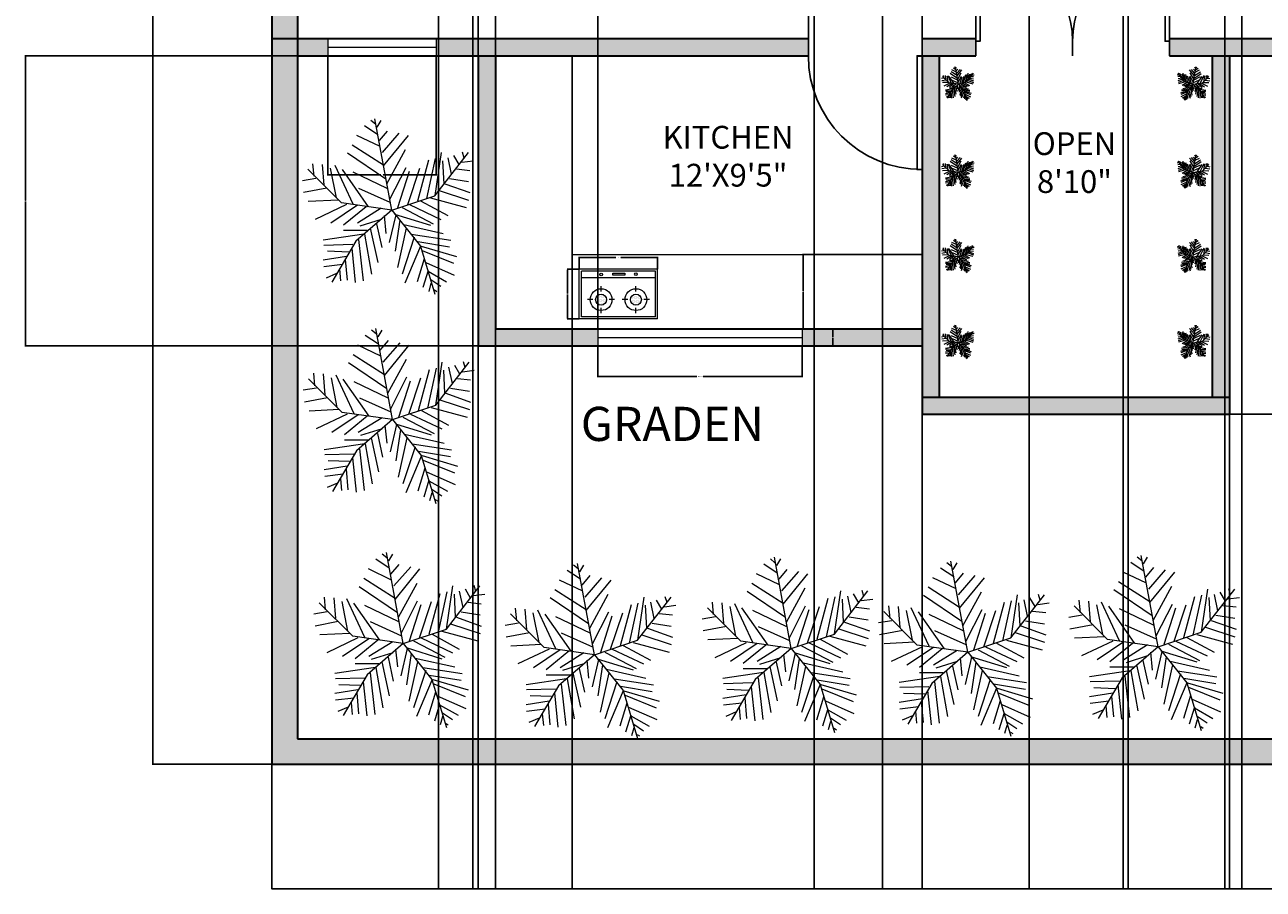
# Model space of a CAD drawing. Units: inches. Extents: x -89 to 661, y -827 to 77.
# Tile 1 of 5: x -89 to 347, y -827 to -523. Entities that reach past the tile are written whole.
import ezdxf

# ---------------------------------------------------------------- set-up
doc = ezdxf.new("R2010")
doc.units = ezdxf.units.IN
doc.header["$MEASUREMENT"] = 0
for name, color, linetype, lineweight in [('A-ANNO-DIMS', 2, 'Continuous', 18), ('A-ANNO-TEXT', 7, 'Continuous', 18), ('A-AREA-IDEN', 7, 'Continuous', 18), ('A-EQPM', 34, 'Continuous', 18), ('A-FLOR-CASE', 34, 'Continuous', 18), ('A-GLAZ', 5, 'Continuous', 18), ('A-WALL', 7, 'Continuous', 35), ('A-WALL-PATT', 30, 'Continuous', 13), ('DOOR', 5, 'Continuous', 25), ('TREE', 3, 'Continuous', 13)]:
    doc.layers.add(name, color=color, linetype=linetype, lineweight=lineweight)
doc.styles.get("Standard").update_dxf_attribs({"font": 'arial.ttf'})
doc.dimstyles.get("Standard").update_dxf_attribs({"dimtxt": 0.18, "dimasz": 0.18, "dimexe": 0.18, "dimexo": 0.0625, "dimgap": 0.09, "dimtad": 0, "dimtih": 1, "dimtoh": 1, "dimdec": 4, "dimzin": 0, "dimdsep": 46, "dimtxsty": 'Standard', "dimcen": 0.09, "dimadec": 0, "dimazin": 0, "dimtfac": 1, "dimtdec": 4, "dimtofl": 0, "dimtmove": 0, "dimatfit": 3, "dimfxl": 1, "dimtolj": 1, "dimtzin": 0, "dimarcsym": 0})

# ---------------------------------------------------------------- blocks, each defined once
blk = doc.blocks.new('*U5')
for p, q in [((-10.186, 53.64), (-13.084, 55.962)), ((0, 0), (-10.5, 57)), ((-9.099, 51.782), (-6.563, 55.962)), ((-7.288, 39.707), (-21.778, 46.673)), ((-8.737, 47.138), (-17.069, 52.711)), ((-7.65, 43.423), (-2.578, 49.46)), ((-5.839, 35.992), (4.667, 48.067)), ((-5.114, 27.632), (10.463, 46.673)), ((-5.114, 28.097), (-24.676, 40.636)), ((-3.665, 19.273), (-27.574, 35.527)), ((-2.941, 16.486), (8.652, 37.85)), ((16.259, 5.805), (23.142, 31.348)), ((22.055, 7.198), (27.489, 32.277)), ((27, 9), (48, 36)), ((27.127, 9.056), (31.112, 35.992)), ((35.096, 32.741), (37.27, 22.524)), ((38.719, 34.134), (41.979, 28.561)), ((44.153, 36.456), (45.239, 32.741)), ((-31.5, 4.5), (-52.5, 25.5)), ((-48.585, 21.131), (-49.309, 29.026)), ((-43.513, 28.561), (-42.427, 15.558)), ((-38.442, 26.239), (-34.819, 7.663)), ((-35.544, 28.097), (-24.314, 3.947)), ((-14.533, 2.09), (-30.834, 25.31)), ((-24.314, 23.917), (-2.941, 13.7)), ((-1.129, 6.734), (9.014, 26.704)), ((3.942, 1.625), (11.187, 24.381)), ((10.101, 3.483), (17.708, 26.239)), ((31.836, 30.883), (32.561, 16.486)), ((40.53, 25.775), (48.862, 24.846)), ((43.791, 29.954), (51.036, 30.883)), ((-47.498, 19.737), (-55.83, 18.344)), ((33.285, 16.486), (48.862, 10.913)), ((36.183, 19.737), (48.137, 17.88)), ((-40.615, 13.7), (-55.105, 10.913)), ((-20.691, 13.7), (-1.129, 4.876)), ((0, 0), (27, 9)), ((29.662, 12.307), (48.137, 6.269)), ((-33.37, 6.269), (-52.207, 5.34)), ((-28.299, 3.483), (-47.86, -5.805)), ((-21.416, 3.018), (-38.079, -8.128)), ((0, 0), (-31.5, 4.5)), ((-15.982, 2.09), (-30.11, -9.521)), ((0, 0), (-22.5, -19.5)), ((-6.563, 1.161), (-21.416, -8.128)), ((0, 0), (18, -22.5)), ((6.478, 1.625), (26.04, -8.592)), ((11.187, 3.483), (30.749, -5.805)), ((18.07, 5.805), (35.096, -3.483)), ((24.229, 7.663), (46.688, 1.625)), ((-6.563, -5.805), (-19.967, -9.985)), ((-4.752, -3.483), (-3.665, -14.629)), ((2.493, -3.019), (-1.491, -20.202)), ((1.769, -2.555), (24.229, -9.521)), ((5.029, -6.27), (2.131, -25.775)), ((-17.431, -15.094), (-42.789, -18.809)), ((-15.257, -12.772), (-30.11, -12.772)), ((-17.069, -15.094), (-12.721, -40.172)), ((-13.446, -11.378), (-8.737, -32.741)), ((-9.461, -8.592), (-6.201, -23.453)), ((9.014, -11.378), (3.58, -35.992)), ((7.565, -9.056), (32.198, -14.629)), ((12.274, -15.094), (36.907, -18.809)), ((-24.314, -21.596), (-42.427, -22.06)), ((-22.5, -19.5), (-37.5, -45)), ((-20.691, -18.345), (-17.793, -44.352)), ((14.085, -16.951), (6.478, -40.172)), ((18.07, -22.524), (8.289, -45.745)), ((16.259, -19.738), (36.183, -22.989)), ((18, -22.5), (27, -52.5)), ((18.433, -22.524), (40.53, -29.026)), ((-28.299, -29.026), (-42.789, -31.348)), ((-26.849, -26.24), (-40.253, -25.775)), ((-29.023, -30.884), (-27.936, -43.887)), ((-25.038, -23.918), (-22.865, -45.281)), ((20.244, -30.419), (15.897, -44.816)), ((19.157, -25.311), (38.719, -33.206)), ((-30.834, -34.135), (-42.427, -35.528)), ((-32.646, -36.921), (-31.921, -44.352)), ((22.78, -37.85), (19.519, -48.532)), ((21.331, -32.741), (39.081, -40.636)), ((22.78, -38.314), (34.372, -44.816)), ((-34.457, -39.708), (-40.978, -42.494)), ((24.591, -45.745), (23.142, -50.854)), ((24.591, -43.423), (30.749, -47.603)), ((26.764, -49.925), (28.213, -50.854))]:
    blk.add_line(p, q)
blk = doc.blocks.new('*U7')
for p, q in [((0, 0), (0, -6)), ((40, 0), (40, -6))]:
    blk.add_line(p, q)
blk.add_lwpolyline([(0, 0), (0, 40), (1.75, 40), (1.75, 0)], close=True)
blk.add_arc((0, 0), 40, 0, 90)
blk = doc.blocks.new('A$C475E21CF')
for p, q in [((0, 444), (0, 0)), ((0, 444), (700, 444)), ((700, 444), (700, 0)), ((19, 425), (19, 19)), ((19, 425), (680, 425)), ((194, 394), (194, 345)), ((505, 394), (505, 345)), ((680, 425), (680, 19)), ((73, 272), (122, 272)), ((149, 264), (149, 264)), ((155, 276), (155, 276)), ((155, 252), (155, 252)), ((161, 288), (161, 288)), ((161, 264), (161, 264)), ((161, 240), (161, 240)), ((167, 301), (167, 301)), ((167, 276), (167, 276)), ((167, 252), (167, 252)), ((173, 288), (173, 288)), ((173, 264), (173, 264)), ((173, 240), (173, 240)), ((179, 301), (179, 301)), ((179, 276), (179, 276)), ((179, 252), (179, 252)), ((179, 228), (179, 228)), ((185, 313), (185, 313)), ((185, 288), (185, 288)), ((185, 264), (185, 264)), ((185, 240), (185, 240)), ((191, 301), (191, 301)), ((191, 276), (191, 276)), ((191, 252), (191, 252)), ((191, 228), (191, 228)), ((197, 313), (197, 313)), ((197, 288), (197, 288)), ((197, 264), (197, 264)), ((197, 240), (197, 240)), ((203, 301), (203, 301)), ((203, 276), (203, 276)), ((203, 252), (203, 252)), ((203, 228), (203, 228)), ((209, 313), (209, 313)), ((209, 288), (209, 288)), ((209, 264), (209, 264)), ((209, 240), (209, 240)), ((216, 301), (216, 301)), ((216, 276), (216, 276)), ((216, 252), (216, 252)), ((216, 228), (216, 228)), ((222, 288), (222, 288)), ((222, 264), (222, 264)), ((222, 240), (222, 240)), ((228, 301), (228, 301)), ((228, 276), (228, 276)), ((228, 252), (228, 252)), ((234, 288), (234, 288)), ((234, 264), (234, 264)), ((234, 240), (234, 240)), ((240, 276), (240, 276)), ((240, 252), (240, 252)), ((267, 272), (316, 272)), ((384, 272), (433, 272)), ((462, 268), (462, 268)), ((468, 280), (468, 280)), ((468, 256), (468, 256)), ((474, 292), (474, 292)), ((474, 268), (474, 268)), ((474, 244), (474, 244)), ((480, 304), (480, 304)), ((480, 280), (480, 280)), ((480, 256), (480, 256)), ((486, 292), (486, 292)), ((486, 268), (486, 268)), ((486, 244), (486, 244)), ((492, 304), (492, 304)), ((492, 280), (492, 280)), ((492, 256), (492, 256)), ((492, 232), (492, 232)), ((498, 317), (498, 317)), ((498, 292), (498, 292)), ((498, 268), (498, 268)), ((498, 244), (498, 244)), ((505, 304), (505, 304)), ((505, 280), (505, 280)), ((505, 256), (505, 256)), ((505, 232), (505, 232)), ((511, 317), (511, 317)), ((511, 292), (511, 292)), ((511, 268), (511, 268)), ((511, 244), (511, 244)), ((517, 304), (517, 304)), ((517, 280), (517, 280)), ((517, 256), (517, 256)), ((517, 232), (517, 232)), ((523, 317), (523, 317)), ((523, 292), (523, 292)), ((523, 268), (523, 268)), ((523, 244), (523, 244)), ((529, 304), (529, 304)), ((529, 280), (529, 280)), ((529, 256), (529, 256)), ((529, 232), (529, 232)), ((535, 292), (535, 292)), ((535, 268), (535, 268)), ((535, 244), (535, 244)), ((541, 304), (541, 304)), ((541, 280), (541, 280)), ((541, 256), (541, 256)), ((547, 292), (547, 292)), ((547, 268), (547, 268)), ((547, 244), (547, 244)), ((553, 280), (553, 280)), ((553, 256), (553, 256)), ((578, 272), (627, 272)), ((194, 199), (194, 151)), ((505, 199), (505, 151)), ((0, 0), (700, 0)), ((19, 78), (680, 78)), ((19, 19), (680, 19)), ((293, 52), (401, 52)), ((293, 36), (293, 52)), ((401, 36), (293, 36)), ((401, 52), (401, 36))]:
    blk.add_line(p, q)
for centre, radius in [((194, 272), 97.2), ((505, 272), 97.2), ((194, 272), 48.6), ((505, 272), 48.6), ((194, 45), 11.7), ((505, 48), 11.7)]:
    blk.add_circle(centre, radius)
blk = doc.blocks.new('WIN-72-NOM')
for p, q in [((0, 6), (0, 0)), ((0, 6), (71.86, 6)), ((71.86, 6), (71.86, 0)), ((0, 3), (71.86, 3)), ((0, 0), (71.86, 0))]:
    blk.add_line(p, q)
blk = doc.blocks.new('*D19')
at = {"layer": 'A-ANNO-DIMS', "color": 0, "lineweight": -2, "transparency": 16777216}
for p, q in [((112.77, -636), (112.77, -646.9)), ((184.63, -636), (184.63, -646.9)), ((112.95, -646.72), (147.58, -646.72)), ((184.45, -646.72), (149.82, -646.72))]:
    blk.add_line(p, q, dxfattribs=at)
at = {"layer": 'A-ANNO-DIMS', "color": 0, "transparency": 16777216}
for points in [[(112.95, -646.69), (112.95, -646.75), (112.77, -646.72)], [(184.45, -646.69), (184.45, -646.75), (184.63, -646.72)]]:
    blk.add_solid(points, dxfattribs=at)
at = {"layer": 'Defpoints', "color": 0, "transparency": 16777216}
for p in [(112.77, -635.94), (184.63, -635.94), (184.63, -646.72)]:
    blk.add_point(p, dxfattribs=at)
at = {"layer": 'A-ANNO-DIMS', "color": 0, "transparency": 16777216, "insert": (148.7, -646.72), "char_height": 0.18, "attachment_point": 5}
blk.add_mtext('\\A1;WINDOW 72 TYP.', dxfattribs=at)
blk = doc.blocks.new('*D20')
at = {"layer": 'A-ANNO-DIMS', "color": 0, "lineweight": -2, "transparency": 16777216}
for p, q in [((184.7, -629.94), (195.59, -629.94)), ((195.41, -630.12), (195.41, -632.76)), ((195.41, -635.76), (195.41, -633.12)), ((184.7, -635.94), (195.59, -635.94))]:
    blk.add_line(p, q, dxfattribs=at)
at = {"layer": 'A-ANNO-DIMS', "color": 0, "transparency": 16777216}
for points in [[(195.38, -630.12), (195.44, -630.12), (195.41, -629.94)], [(195.38, -635.76), (195.44, -635.76), (195.41, -635.94)]]:
    blk.add_solid(points, dxfattribs=at)
at = {"layer": 'Defpoints', "color": 0, "transparency": 16777216}
for p in [(184.63, -629.94), (195.41, -629.94), (184.63, -635.94)]:
    blk.add_point(p, dxfattribs=at)
at = {"layer": 'A-ANNO-DIMS', "color": 0, "transparency": 16777216, "insert": (195.41, -632.94), "char_height": 0.18, "attachment_point": 5}
blk.add_mtext('\\A1;6 TYP.', dxfattribs=at)
blk = doc.blocks.new('*D29')
at = {"layer": 'A-ANNO-DIMS', "color": 0, "lineweight": -2, "transparency": 16777216}
for p, q in [((106.27, -608.89), (106.27, -604.64)), ((106.45, -604.82), (119.17, -604.82)), ((133.64, -604.82), (120.93, -604.82)), ((133.82, -608.89), (133.82, -604.64))]:
    blk.add_line(p, q, dxfattribs=at)
at = {"layer": 'A-ANNO-DIMS', "color": 0, "transparency": 16777216}
for points in [[(106.45, -604.79), (106.45, -604.85), (106.27, -604.82)], [(133.64, -604.79), (133.64, -604.85), (133.82, -604.82)]]:
    blk.add_solid(points, dxfattribs=at)
at = {"layer": 'Defpoints', "color": 0, "transparency": 16777216}
for p in [(106.27, -604.82), (106.27, -608.95), (133.82, -608.95)]:
    blk.add_point(p, dxfattribs=at)
at = {"layer": 'A-ANNO-DIMS', "color": 0, "transparency": 16777216, "insert": (120.05, -604.82), "char_height": 0.18, "attachment_point": 5}
blk.add_mtext('\\A1;COOKTOP 28', dxfattribs=at)
blk = doc.blocks.new('*D30')
at = {"layer": 'A-ANNO-DIMS', "color": 0, "lineweight": -2, "transparency": 16777216}
for p, q in [((106.21, -608.95), (101.96, -608.95)), ((102.14, -609.13), (102.14, -617.52)), ((102.14, -626.27), (102.14, -617.88)), ((106.21, -626.45), (101.96, -626.45))]:
    blk.add_line(p, q, dxfattribs=at)
at = {"layer": 'A-ANNO-DIMS', "color": 0, "transparency": 16777216}
for points in [[(102.11, -609.13), (102.17, -609.13), (102.14, -608.95)], [(102.11, -626.27), (102.17, -626.27), (102.14, -626.45)]]:
    blk.add_solid(points, dxfattribs=at)
at = {"layer": 'Defpoints', "color": 0, "transparency": 16777216}
for p in [(106.27, -608.95), (102.14, -626.45), (106.27, -626.45)]:
    blk.add_point(p, dxfattribs=at)
at = {"layer": 'A-ANNO-DIMS', "color": 0, "transparency": 16777216, "insert": (102.14, -617.7), "char_height": 0.18, "attachment_point": 5}
blk.add_mtext('\\A1;17', dxfattribs=at)
blk = doc.blocks.new('*D31')
at = {"layer": 'A-ANNO-DIMS', "color": 0, "lineweight": -2, "transparency": 16777216}
for p, q in [((-1.81, -783), (-1.81, -826.85)), ((619.19, -783), (619.19, -826.85)), ((-1.63, -826.67), (308.41, -826.67)), ((619.01, -826.67), (308.96, -826.67))]:
    blk.add_line(p, q, dxfattribs=at)
at = {"layer": 'A-ANNO-DIMS', "color": 0, "transparency": 16777216}
for points in [[(-1.63, -826.64), (-1.63, -826.7), (-1.81, -826.67)], [(619.01, -826.64), (619.01, -826.7), (619.19, -826.67)]]:
    blk.add_solid(points, dxfattribs=at)
at = {"layer": 'Defpoints', "color": 0, "transparency": 16777216}
for p in [(-1.81, -782.94), (619.19, -782.94), (619.19, -826.67)]:
    blk.add_point(p, dxfattribs=at)
at = {"layer": 'A-ANNO-DIMS', "color": 0, "transparency": 16777216, "insert": (308.69, -826.67), "char_height": 0.18, "attachment_point": 5}
blk.add_mtext('\\A1;621', dxfattribs=at)
blk = doc.blocks.new('*D32')
at = {"layer": 'A-ANNO-DIMS', "color": 0, "lineweight": -2, "transparency": 16777216}
for p, q in [((-1.88, 29.06), (-43.85, 29.06)), ((-43.67, 28.88), (-43.67, -376.76)), ((-43.67, -782.76), (-43.67, -377.12)), ((-1.88, -782.94), (-43.85, -782.94))]:
    blk.add_line(p, q, dxfattribs=at)
at = {"layer": 'A-ANNO-DIMS', "color": 0, "transparency": 16777216}
for points in [[(-43.7, 28.88), (-43.64, 28.88), (-43.67, 29.06)], [(-43.7, -782.76), (-43.64, -782.76), (-43.67, -782.94)]]:
    blk.add_solid(points, dxfattribs=at)
at = {"layer": 'Defpoints', "color": 0, "transparency": 16777216}
for p in [(-43.67, 29.06), (-1.81, 29.06), (-1.81, -782.94)]:
    blk.add_point(p, dxfattribs=at)
at = {"layer": 'A-ANNO-DIMS', "color": 0, "transparency": 16777216, "insert": (-43.67, -376.94), "char_height": 0.18, "attachment_point": 5}
blk.add_mtext('\\A1;812', dxfattribs=at)
blk = doc.blocks.new('*D44')
at = {"layer": 'A-ANNO-DIMS', "color": 0, "lineweight": -2, "transparency": 16777216}
for p, q in [((299.19, -34), (299.19, -826.85)), ((333.19, -34), (333.19, -826.85)), ((299.37, -826.67), (315.97, -826.67)), ((333.01, -826.67), (316.4, -826.67))]:
    blk.add_line(p, q, dxfattribs=at)
at = {"layer": 'A-ANNO-DIMS', "color": 0, "transparency": 16777216}
for points in [[(299.37, -826.64), (299.37, -826.7), (299.19, -826.67)], [(333.01, -826.64), (333.01, -826.7), (333.19, -826.67)]]:
    blk.add_solid(points, dxfattribs=at)
at = {"layer": 'Defpoints', "color": 0, "transparency": 16777216}
for p in [(299.19, -33.94), (333.19, -33.94), (333.19, -826.67)]:
    blk.add_point(p, dxfattribs=at)
at = {"layer": 'A-ANNO-DIMS', "color": 0, "transparency": 16777216, "insert": (316.19, -826.67), "char_height": 0.18, "attachment_point": 5}
blk.add_mtext('\\A1;34', dxfattribs=at)
blk = doc.blocks.new('*D46')
at = {"layer": 'A-ANNO-DIMS', "color": 0, "lineweight": -2, "transparency": 16777216}
for p, q in [((333.19, -34), (333.19, -826.85)), ((339.19, -34), (339.19, -826.85)), ((333.37, -826.67), (336.04, -826.67)), ((339.01, -826.67), (336.34, -826.67))]:
    blk.add_line(p, q, dxfattribs=at)
at = {"layer": 'A-ANNO-DIMS', "color": 0, "transparency": 16777216}
for points in [[(333.37, -826.64), (333.37, -826.7), (333.19, -826.67)], [(339.01, -826.64), (339.01, -826.7), (339.19, -826.67)]]:
    blk.add_solid(points, dxfattribs=at)
at = {"layer": 'Defpoints', "color": 0, "transparency": 16777216}
for p in [(333.19, -33.94), (339.19, -33.94), (339.19, -826.67)]:
    blk.add_point(p, dxfattribs=at)
at = {"layer": 'A-ANNO-DIMS', "color": 0, "transparency": 16777216, "insert": (336.19, -826.67), "char_height": 0.18, "attachment_point": 5}
blk.add_mtext('\\A1;6', dxfattribs=at)
blk = doc.blocks.new('*D48')
at = {"layer": 'A-ANNO-DIMS', "color": 0, "lineweight": -2, "transparency": 16777216}
for p, q in [((297.44, 2.03), (297.44, -826.85)), ((264.44, -8.47), (264.44, -826.85)), ((264.62, -826.67), (280.72, -826.67)), ((297.26, -826.67), (281.15, -826.67))]:
    blk.add_line(p, q, dxfattribs=at)
at = {"layer": 'A-ANNO-DIMS', "color": 0, "transparency": 16777216}
for points in [[(264.62, -826.64), (264.62, -826.7), (264.44, -826.67)], [(297.26, -826.64), (297.26, -826.7), (297.44, -826.67)]]:
    blk.add_solid(points, dxfattribs=at)
at = {"layer": 'Defpoints', "color": 0, "transparency": 16777216}
for p in [(297.44, 2.09), (264.44, -8.41), (297.44, -826.67)]:
    blk.add_point(p, dxfattribs=at)
at = {"layer": 'A-ANNO-DIMS', "color": 0, "transparency": 16777216, "insert": (280.94, -826.67), "char_height": 0.18, "attachment_point": 5}
blk.add_mtext('\\A1;33', dxfattribs=at)
blk = doc.blocks.new('*D55')
at = {"layer": 'A-ANNO-DIMS', "color": 0, "lineweight": -2, "transparency": 16777216}
for p, q in [((56.84, -267), (56.84, -826.85)), ((68.84, -267), (68.84, -826.85)), ((57.02, -826.67), (62.63, -826.67)), ((68.66, -826.67), (63.05, -826.67))]:
    blk.add_line(p, q, dxfattribs=at)
at = {"layer": 'A-ANNO-DIMS', "color": 0, "transparency": 16777216}
for points in [[(57.02, -826.64), (57.02, -826.7), (56.84, -826.67)], [(68.66, -826.64), (68.66, -826.7), (68.84, -826.67)]]:
    blk.add_solid(points, dxfattribs=at)
at = {"layer": 'Defpoints', "color": 0, "transparency": 16777216}
for p in [(56.84, -266.94), (68.84, -266.94), (68.84, -826.67)]:
    blk.add_point(p, dxfattribs=at)
at = {"layer": 'A-ANNO-DIMS', "color": 0, "transparency": 16777216, "insert": (62.84, -826.67), "char_height": 0.18, "attachment_point": 5}
blk.add_mtext('\\A1;12', dxfattribs=at)
blk = doc.blocks.new('*D56')
at = {"layer": 'A-ANNO-DIMS', "color": 0, "lineweight": -2, "transparency": 16777216}
for p, q in [((188.84, -312), (188.84, -826.85)), ((212.84, -318), (212.84, -826.85)), ((189.02, -826.67), (200.62, -826.67)), ((212.66, -826.67), (201.06, -826.67))]:
    blk.add_line(p, q, dxfattribs=at)
at = {"layer": 'A-ANNO-DIMS', "color": 0, "transparency": 16777216}
for points in [[(189.02, -826.64), (189.02, -826.7), (188.84, -826.67)], [(212.66, -826.64), (212.66, -826.7), (212.84, -826.67)]]:
    blk.add_solid(points, dxfattribs=at)
at = {"layer": 'Defpoints', "color": 0, "transparency": 16777216}
for p in [(188.84, -311.94), (212.84, -317.94), (212.84, -826.67)]:
    blk.add_point(p, dxfattribs=at)
at = {"layer": 'A-ANNO-DIMS', "color": 0, "transparency": 16777216, "insert": (200.84, -826.67), "char_height": 0.18, "attachment_point": 5}
blk.add_mtext('\\A1;24', dxfattribs=at)
blk = doc.blocks.new('*D57')
at = {"layer": 'A-ANNO-DIMS', "color": 0, "lineweight": -2, "transparency": 16777216}
for p, q in [((70.79, -636), (70.79, -826.85)), ((226.79, -636), (226.79, -826.85)), ((70.97, -826.67), (148.51, -826.67)), ((226.61, -826.67), (149.07, -826.67))]:
    blk.add_line(p, q, dxfattribs=at)
at = {"layer": 'A-ANNO-DIMS', "color": 0, "transparency": 16777216}
for points in [[(70.97, -826.64), (70.97, -826.7), (70.79, -826.67)], [(226.61, -826.64), (226.61, -826.7), (226.79, -826.67)]]:
    blk.add_solid(points, dxfattribs=at)
at = {"layer": 'Defpoints', "color": 0, "transparency": 16777216}
for p in [(70.79, -635.94), (226.79, -635.94), (226.79, -826.67)]:
    blk.add_point(p, dxfattribs=at)
at = {"layer": 'A-ANNO-DIMS', "color": 0, "transparency": 16777216, "insert": (148.79, -826.67), "char_height": 0.18, "attachment_point": 5}
blk.add_mtext('\\A1;156', dxfattribs=at)
blk = doc.blocks.new('*D58')
at = {"layer": 'A-ANNO-DIMS', "color": 0, "lineweight": -2, "transparency": 16777216}
for p, q in [((226.79, -660), (226.79, -826.85)), ((334.79, -660), (334.79, -826.85)), ((226.97, -826.67), (280.51, -826.67)), ((334.61, -826.67), (281.07, -826.67))]:
    blk.add_line(p, q, dxfattribs=at)
at = {"layer": 'A-ANNO-DIMS', "color": 0, "transparency": 16777216}
for points in [[(226.97, -826.64), (226.97, -826.7), (226.79, -826.67)], [(334.61, -826.64), (334.61, -826.7), (334.79, -826.67)]]:
    blk.add_solid(points, dxfattribs=at)
at = {"layer": 'Defpoints', "color": 0, "transparency": 16777216}
for p in [(226.79, -659.94), (334.79, -659.94), (334.79, -826.67)]:
    blk.add_point(p, dxfattribs=at)
at = {"layer": 'A-ANNO-DIMS', "color": 0, "transparency": 16777216, "insert": (280.79, -826.67), "char_height": 0.18, "attachment_point": 5}
blk.add_mtext('\\A1;108', dxfattribs=at)
blk = doc.blocks.new('*D59')
at = {"layer": 'A-ANNO-DIMS', "color": 0, "lineweight": -2, "transparency": 16777216}
for p, q in [((70.73, -533.94), (-88.61, -533.94)), ((-88.43, -534.12), (-88.43, -584.76)), ((-88.43, -635.76), (-88.43, -585.12)), ((70.73, -635.94), (-88.61, -635.94))]:
    blk.add_line(p, q, dxfattribs=at)
at = {"layer": 'A-ANNO-DIMS', "color": 0, "transparency": 16777216}
for points in [[(-88.46, -534.12), (-88.4, -534.12), (-88.43, -533.94)], [(-88.46, -635.76), (-88.4, -635.76), (-88.43, -635.94)]]:
    blk.add_solid(points, dxfattribs=at)
at = {"layer": 'Defpoints', "color": 0, "transparency": 16777216}
for p in [(-88.43, -533.94), (70.79, -533.94), (70.79, -635.94)]:
    blk.add_point(p, dxfattribs=at)
at = {"layer": 'A-ANNO-DIMS', "color": 0, "transparency": 16777216, "insert": (-88.43, -584.94), "char_height": 0.18, "attachment_point": 5}
blk.add_mtext('\\A1;102', dxfattribs=at)
blk = doc.blocks.new('*D60')
at = {"layer": 'A-ANNO-DIMS', "color": 0, "lineweight": -2, "transparency": 16777216}
for p, q in [((334.85, -533.94), (661.23, -533.94)), ((661.05, -534.12), (661.05, -596.76)), ((661.05, -659.76), (661.05, -597.12)), ((334.85, -659.94), (661.23, -659.94))]:
    blk.add_line(p, q, dxfattribs=at)
at = {"layer": 'A-ANNO-DIMS', "color": 0, "transparency": 16777216}
for points in [[(661.02, -534.12), (661.08, -534.12), (661.05, -533.94)], [(661.02, -659.76), (661.08, -659.76), (661.05, -659.94)]]:
    blk.add_solid(points, dxfattribs=at)
at = {"layer": 'Defpoints', "color": 0, "transparency": 16777216}
for p in [(334.79, -533.94), (661.05, -533.94), (334.79, -659.94)]:
    blk.add_point(p, dxfattribs=at)
at = {"layer": 'A-ANNO-DIMS', "color": 0, "transparency": 16777216, "insert": (661.05, -596.94), "char_height": 0.18, "attachment_point": 5}
blk.add_mtext('\\A1;126', dxfattribs=at)
blk = doc.blocks.new('*D62')
at = {"layer": 'A-ANNO-DIMS', "color": 0, "lineweight": -2, "transparency": 16777216}
for p, q in [((186.79, -527.88), (186.79, 77.13)), ((186.97, 76.95), (206.57, 76.95)), ((226.61, 76.95), (207.01, 76.95)), ((226.79, -527.88), (226.79, 77.13))]:
    blk.add_line(p, q, dxfattribs=at)
at = {"layer": 'A-ANNO-DIMS', "color": 0, "transparency": 16777216}
for points in [[(186.97, 76.98), (186.97, 76.92), (186.79, 76.95)], [(226.61, 76.98), (226.61, 76.92), (226.79, 76.95)]]:
    blk.add_solid(points, dxfattribs=at)
at = {"layer": 'Defpoints', "color": 0, "transparency": 16777216}
for p in [(226.79, 76.95), (186.79, -527.94), (226.79, -527.94)]:
    blk.add_point(p, dxfattribs=at)
at = {"layer": 'A-ANNO-DIMS', "color": 0, "transparency": 16777216, "insert": (206.79, 76.95), "char_height": 0.18, "attachment_point": 5}
blk.add_mtext('\\A1;40', dxfattribs=at)
blk = doc.blocks.new('*D63')
at = {"layer": 'A-ANNO-DIMS', "color": 0, "lineweight": -2, "transparency": 16777216}
for p, q in [((7.19, -533.88), (7.19, -491.9)), ((70.79, -533.88), (70.79, -491.9)), ((7.37, -492.08), (38.66, -492.08)), ((70.61, -492.08), (39.31, -492.08))]:
    blk.add_line(p, q, dxfattribs=at)
at = {"layer": 'A-ANNO-DIMS', "color": 0, "transparency": 16777216}
for points in [[(7.37, -492.05), (7.37, -492.11), (7.19, -492.08)], [(70.61, -492.05), (70.61, -492.11), (70.79, -492.08)]]:
    blk.add_solid(points, dxfattribs=at)
at = {"layer": 'Defpoints', "color": 0, "transparency": 16777216}
for p in [(70.79, -492.08), (7.19, -533.94), (70.79, -533.94)]:
    blk.add_point(p, dxfattribs=at)
at = {"layer": 'A-ANNO-DIMS', "color": 0, "transparency": 16777216, "insert": (38.99, -492.08), "char_height": 0.18, "attachment_point": 5}
blk.add_mtext('\\A1;63.6', dxfattribs=at)
blk = doc.blocks.new('*D66')
at = {"layer": 'A-ANNO-DIMS', "color": 0, "lineweight": -2, "transparency": 16777216}
for p, q in [((17.9, -534), (17.9, -575.98)), ((55.96, -534), (55.96, -575.98)), ((18.08, -575.8), (36.54, -575.8)), ((55.78, -575.8), (37.33, -575.8))]:
    blk.add_line(p, q, dxfattribs=at)
at = {"layer": 'A-ANNO-DIMS', "color": 0, "transparency": 16777216}
for points in [[(18.08, -575.77), (18.08, -575.83), (17.9, -575.8)], [(55.78, -575.77), (55.78, -575.83), (55.96, -575.8)]]:
    blk.add_solid(points, dxfattribs=at)
at = {"layer": 'Defpoints', "color": 0, "transparency": 16777216}
for p in [(17.9, -533.94), (55.96, -533.94), (17.9, -575.8)]:
    blk.add_point(p, dxfattribs=at)
at = {"layer": 'A-ANNO-DIMS', "color": 0, "transparency": 16777216, "insert": (36.93, -575.8), "char_height": 0.18, "attachment_point": 5}
blk.add_mtext('\\A1;38.06', dxfattribs=at)
blk = doc.blocks.new('*D67')
at = {"layer": 'A-ANNO-DIMS', "color": 0, "lineweight": -2, "transparency": 16777216}
for p, q in [((226.73, -603.76), (184.75, -603.76)), ((184.93, -603.94), (184.93, -616.67)), ((184.93, -629.76), (184.93, -617.03)), ((226.73, -629.94), (184.75, -629.94))]:
    blk.add_line(p, q, dxfattribs=at)
at = {"layer": 'A-ANNO-DIMS', "color": 0, "transparency": 16777216}
for points in [[(184.9, -603.94), (184.96, -603.94), (184.93, -603.76)], [(184.9, -629.76), (184.96, -629.76), (184.93, -629.94)]]:
    blk.add_solid(points, dxfattribs=at)
at = {"layer": 'Defpoints', "color": 0, "transparency": 16777216}
for p in [(184.93, -603.76), (226.79, -603.76), (226.79, -629.94)]:
    blk.add_point(p, dxfattribs=at)
at = {"layer": 'A-ANNO-DIMS', "color": 0, "transparency": 16777216, "insert": (184.93, -616.85), "char_height": 0.18, "attachment_point": 5}
blk.add_mtext('\\A1;26.18', dxfattribs=at)
blk = doc.blocks.new('*D68')
at = {"layer": 'A-ANNO-DIMS', "color": 0, "lineweight": -2, "transparency": 16777216}
for p, q in [((76.79, -534), (76.79, -826.85)), ((103.81, -534), (103.81, -826.85)), ((76.97, -826.67), (89.9, -826.67)), ((103.63, -826.67), (90.69, -826.67))]:
    blk.add_line(p, q, dxfattribs=at)
at = {"layer": 'A-ANNO-DIMS', "color": 0, "transparency": 16777216}
for points in [[(76.97, -826.64), (76.97, -826.7), (76.79, -826.67)], [(103.63, -826.64), (103.63, -826.7), (103.81, -826.67)]]:
    blk.add_solid(points, dxfattribs=at)
at = {"layer": 'Defpoints', "color": 0, "transparency": 16777216}
for p in [(76.79, -533.94), (103.81, -533.94), (103.81, -826.67)]:
    blk.add_point(p, dxfattribs=at)
at = {"layer": 'A-ANNO-DIMS', "color": 0, "transparency": 16777216, "insert": (90.3, -826.67), "char_height": 0.18, "attachment_point": 5}
blk.add_mtext('\\A1;27.02', dxfattribs=at)
blk = doc.blocks.new('*D69')
at = {"layer": 'A-ANNO-DIMS', "color": 0, "lineweight": -2, "transparency": 16777216}
for p, q in [((76.79, -629.88), (76.79, 77.13)), ((76.97, 76.95), (94.39, 76.95)), ((112.59, 76.95), (95.17, 76.95)), ((112.77, -629.88), (112.77, 77.13))]:
    blk.add_line(p, q, dxfattribs=at)
at = {"layer": 'A-ANNO-DIMS', "color": 0, "transparency": 16777216}
for points in [[(76.97, 76.98), (76.97, 76.92), (76.79, 76.95)], [(112.59, 76.98), (112.59, 76.92), (112.77, 76.95)]]:
    blk.add_solid(points, dxfattribs=at)
at = {"layer": 'Defpoints', "color": 0, "transparency": 16777216}
for p in [(112.77, 76.95), (76.79, -629.94), (112.77, -629.94)]:
    blk.add_point(p, dxfattribs=at)
at = {"layer": 'A-ANNO-DIMS', "color": 0, "transparency": 16777216, "insert": (94.78, 76.95), "char_height": 0.18, "attachment_point": 5}
blk.add_mtext('\\A1;35.98', dxfattribs=at)
blk = doc.blocks.new('*D74')
at = {"layer": 'A-ANNO-DIMS', "color": 0, "lineweight": -2, "transparency": 16777216}
for p, q in [((313.68, -527.88), (313.68, -485.9)), ((313.86, -486.08), (351.48, -486.08)), ((389.89, -486.08), (352.27, -486.08)), ((390.07, -527.88), (390.07, -485.9))]:
    blk.add_line(p, q, dxfattribs=at)
at = {"layer": 'A-ANNO-DIMS', "color": 0, "transparency": 16777216}
for points in [[(313.86, -486.05), (313.86, -486.11), (313.68, -486.08)], [(389.89, -486.05), (389.89, -486.11), (390.07, -486.08)]]:
    blk.add_solid(points, dxfattribs=at)
at = {"layer": 'Defpoints', "color": 0, "transparency": 16777216}
for p in [(390.07, -486.08), (313.68, -527.94), (390.07, -527.94)]:
    blk.add_point(p, dxfattribs=at)
at = {"layer": 'A-ANNO-DIMS', "color": 0, "transparency": 16777216, "insert": (351.88, -486.08), "char_height": 0.18, "attachment_point": 5}
blk.add_mtext('\\A1;76.39', dxfattribs=at)

msp = doc.modelspace()

# ---------------------------------------------------------------- hatches: boundary and pattern name
at = {"layer": 'A-WALL-PATT'}
h = msp.add_hatch(color=256, dxfattribs=at)
h.dxf.hatch_style = 1
h.paths.add_polyline_path([(255.186, 29.06), (-1.814, 29.06), (-1.814, -33.94), (7.186, -33.94), (7.186, -27.94), (7.186, 20.06), (255.186, 20.06)])
h.paths.add_polyline_path([(174.616, -27.94), (7.186, -27.94), (7.186, -33.94), (174.616, -33.94)], flags=17)
h.paths.add_polyline_path([(7.186, -33.94), (-1.814, -33.94), (-1.814, -527.94), (7.186, -527.94), (7.186, -425.94), (7.186, -311.94), (7.186, -207.94)])
h.paths.add_polyline_path([(7.186, -527.94), (-1.814, -527.94), (-1.814, -782.94), (430.186, -782.94), (430.186, -773.94), (7.186, -773.94)])
h = msp.add_hatch(color=256, dxfattribs=at)
h.dxf.hatch_style = 1
h.paths.add_polyline_path([(619.186, -533.94), (610.186, -533.94), (610.186, -773.94), (610.186, -782.94), (619.186, -782.94)])
h.paths.add_polyline_path([(610.186, -527.94), (461.934, -527.94), (461.934, -533.94), (610.186, -533.94)])
h.paths.add_polyline_path([(390.071, -527.94), (313.682, -527.94), (313.682, -528.84), (313.682, -533.94), (390.071, -533.94)])
h.paths.add_polyline_path([(334.788, -533.94), (328.788, -533.94), (328.788, -653.94), (334.788, -653.94)])
h.paths.add_polyline_path([(334.788, -653.94), (226.788, -653.94), (226.788, -659.94), (334.788, -659.94)])
h.paths.add_polyline_path([(232.788, -533.94), (226.788, -533.94), (226.788, -573.94), (226.788, -653.94), (232.788, -653.94)])
h.paths.add_polyline_path([(245.682, -528.84), (245.682, -527.94), (226.788, -527.94), (226.788, -533.94), (232.788, -533.94), (245.682, -533.94)])
h.paths.add_polyline_path([(226.788, -629.94), (184.634, -629.94), (184.634, -635.94), (226.788, -635.94)])
h.paths.add_polyline_path([(76.788, -533.94), (70.788, -533.94), (70.788, -635.94), (112.77, -635.94), (112.77, -629.94), (76.788, -629.94)])
h.paths.add_polyline_path([(186.788, -527.94), (55.963, -527.94), (55.963, -533.94), (186.788, -533.94)])
h.paths.add_polyline_path([(17.901, -527.94), (7.186, -527.94), (7.186, -533.94), (17.901, -533.94)])

# ---------------------------------------------------------------- linework, layer by layer
at = {"layer": 'A-FLOR-CASE'}
for p, q in [((103.806, -533.94), (103.806, -603.761)), ((103.806, -603.761), (226.788, -603.761))]:
    msp.add_line(p, q, dxfattribs=at)
at = {"layer": 'A-GLAZ'}
for p, q in [((17.901, -527.94), (17.901, -533.94)), ((17.901, -527.94), (55.963, -527.94)), ((17.901, -530.94), (55.963, -530.94)), ((55.963, -527.94), (55.963, -533.94)), ((17.901, -533.94), (55.963, -533.94))]:
    msp.add_line(p, q, dxfattribs=at)
at = {"layer": 'A-WALL'}
for p, q in [((-1.814, 29.06), (-1.814, -782.94)), ((7.186, -425.94), (7.186, -527.94)), ((-1.814, -527.94), (186.788, -527.94)), ((7.186, -527.94), (7.186, -773.94)), ((226.788, -527.94), (245.682, -527.94)), ((279.677, -527.94), (279.694, -527.94)), ((313.682, -527.94), (610.186, -527.94)), ((7.186, -533.94), (186.788, -533.94)), ((70.788, -533.94), (70.788, -635.94)), ((76.788, -533.94), (76.788, -629.94)), ((225.038, -533.94), (245.682, -533.94)), ((226.788, -533.94), (226.788, -659.94)), ((232.788, -533.94), (232.788, -653.94)), ((313.682, -533.94), (619.186, -533.94)), ((328.788, -533.94), (328.788, -653.94)), ((334.788, -533.94), (334.788, -659.94)), ((76.788, -629.94), (226.788, -629.94)), ((70.788, -635.94), (226.788, -635.94)), ((226.788, -653.94), (334.788, -653.94)), ((226.788, -659.94), (334.788, -659.94)), ((7.186, -773.94), (430.186, -773.94)), ((-1.814, -782.94), (430.186, -782.94))]:
    msp.add_line(p, q, dxfattribs=at)

# ---------------------------------------------------------------- block references
at = {"layer": 'A-EQPM', "xscale": 0.0393700787401575, "yscale": 0.0393700787401575, "zscale": 0.0393700787401575, "rotation": 180}
msp.add_blockref('A$C475E21CF', (133.825, -608.954), dxfattribs=at)
at = {"layer": 'A-GLAZ'}
msp.add_blockref('WIN-72-NOM', (112.77, -635.94), dxfattribs=at)
at = {"layer": 'DOOR', "yscale": 0.85, "zscale": 0.85}
for p, xscale in [((245.682, -528.84), 0.85), ((313.682, -528.84), -0.85)]:
    msp.add_blockref('*U7', p, dxfattribs=dict(at, xscale=xscale))
at = {"layer": 'DOOR', "rotation": 180}
msp.add_blockref('*U7', (226.788, -533.94), dxfattribs=at)
at = {"layer": 'TREE'}
for p, xscale, yscale, zscale in [((239.628, -543.971), 0.1077469548948497, 0.1077469548948497, 0.1077469548948497), ((321.948, -543.971), -0.1077469548948497, 0.1077469548948497, 0.1077469548948497), ((40.335, -588.179), 0.5618197724328321, 0.5618197724328321, 0.5618197724328321), ((239.628, -574.919), 0.1077469548948497, 0.1077469548948497, 0.1077469548948497), ((321.948, -574.919), -0.1077469548948497, 0.1077469548948497, 0.1077469548948497), ((239.628, -604.573), 0.1077469548948497, 0.1077469548948497, 0.1077469548948497), ((321.948, -604.573), -0.1077469548948497, 0.1077469548948497, 0.1077469548948497), ((40.64, -661.832), 0.5618197724328321, 0.5618197724328321, 0.5618197724328321), ((239.628, -634.78), 0.1077469548948497, 0.1077469548948497, 0.1077469548948497), ((321.948, -634.78), -0.1077469548948497, 0.1077469548948497, 0.1077469548948497), ((44.391, -740.505), 0.5618197724328321, 0.5618197724328321, 0.5618197724328321), ((111.587, -744.422), 0.5618197724328321, 0.5618197724328321, 0.5618197724328321), ((180.785, -742.232), 0.5618197724328321, 0.5618197724328321, 0.5618197724328321), ((242.796, -743.587), 0.5618197724328321, 0.5618197724328321, 0.5618197724328321), ((309.698, -741.627), 0.5618197724328321, 0.5618197724328321, 0.5618197724328321)]:
    msp.add_blockref('*U5', p, dxfattribs=dict(at, xscale=xscale, yscale=yscale, zscale=zscale))

# ---------------------------------------------------------------- texts
at = {"layer": 'A-ANNO-TEXT', "insert": (110.851, -657.321), "char_height": 12, "attachment_point": 1}
msp.add_mtext_dynamic_manual_height_columns('\\pxqc;{\\fArial|b1|i0|c0|p34;GRADEN}', width=56.29646, gutter_width=1, heights=[0], dxfattribs=at)
at = {"layer": 'A-AREA-IDEN', "char_height": 8, "attachment_point": 1}
for s, insert in [('\\pxqc;KITCHEN\\P12\'X9\'5"', (130.425, -558.585)), ('\\pxqc;OPEN\\P8\'10"', (252.176, -560.836))]:
    msp.add_mtext_dynamic_manual_height_columns(s, width=56.29646, gutter_width=1, heights=[0], dxfattribs=dict(at, insert=insert))

# ---------------------------------------------------------------- dimensions: what is measured, and where the dimension line sits
at = {"layer": 'A-ANNO-DIMS'}
for base, p1, p2, override, picture, middle in [((112.77, 76.952), (76.788, -629.94), (112.77, -629.94), {"dimdec": 2, "dimlfac": 1, "dimrnd": 0, "dimzin": 0, "dimdsep": 46, "dimlunit": 2}, '*D69', (94.779, 76.952)), ((226.788, 76.952), (186.788, -527.94), (226.788, -527.94), {"dimdec": 0, "dimlfac": 1, "dimrnd": 0, "dimzin": 0, "dimdsep": 46, "dimlunit": 2}, '*D62', (206.788, 76.952)), ((297.436, -826.669), (264.436, -8.408), (297.436, 2.092), {"dimdec": 0, "dimlfac": 1, "dimrnd": 0, "dimzin": 0, "dimdsep": 46, "dimlunit": 2}, '*D48', (280.936, -826.669)), ((333.186, -826.669), (299.186, -33.94), (333.186, -33.94), {"dimdec": 0, "dimlfac": 1, "dimrnd": 0, "dimzin": 0, "dimdsep": 46, "dimlunit": 2}, '*D44', (316.186, -826.669)), ((339.186, -826.669), (333.186, -33.94), (339.186, -33.94), {"dimdec": 0, "dimlfac": 1, "dimrnd": 0, "dimzin": 0, "dimdsep": 46, "dimlunit": 2}, '*D46', (336.186, -826.669)), ((68.837, -826.669), (56.837, -266.94), (68.837, -266.94), {"dimdec": 0, "dimlfac": 1, "dimrnd": 0, "dimzin": 0, "dimdsep": 46, "dimlunit": 2}, '*D55', (62.837, -826.669)), ((212.837, -826.669), (188.837, -311.94), (212.837, -317.94), {"dimdec": 0, "dimlfac": 1, "dimrnd": 0, "dimzin": 0, "dimdsep": 46, "dimlunit": 2}, '*D56', (200.837, -826.669)), ((390.071, -486.08), (313.682, -527.94), (390.071, -527.94), {"dimdec": 2, "dimlfac": 1, "dimrnd": 0, "dimzin": 0, "dimdsep": 46, "dimlunit": 2}, '*D74', (351.876, -486.08)), ((70.788, -492.08), (7.186, -533.94), (70.788, -533.94), {"dimdec": 1, "dimlfac": 1, "dimrnd": 0, "dimzin": 0, "dimdsep": 46, "dimlunit": 2}, '*D63', (38.987, -492.08)), ((103.806, -826.669), (76.788, -533.94), (103.806, -533.94), {"dimdec": 2, "dimlfac": 1, "dimrnd": 0, "dimzin": 0, "dimdsep": 46, "dimlunit": 2}, '*D68', (90.297, -826.669)), ((226.788, -826.669), (70.788, -635.94), (226.788, -635.94), {"dimdec": 0, "dimlfac": 1, "dimrnd": 0, "dimzin": 0, "dimdsep": 46, "dimlunit": 2}, '*D57', (148.788, -826.669)), ((334.788, -826.669), (226.788, -659.94), (334.788, -659.94), {"dimdec": 0, "dimlfac": 1, "dimrnd": 0, "dimzin": 0, "dimdsep": 46, "dimlunit": 2}, '*D58', (280.788, -826.669)), ((619.186, -826.669), (-1.814, -782.94), (619.186, -782.94), {"dimdec": 0, "dimlfac": 1, "dimrnd": 0, "dimzin": 0, "dimdsep": 46, "dimlunit": 2}, '*D31', (308.686, -826.669))]:
    dim = msp.add_linear_dim(base=base, p1=p1, p2=p2, dimstyle='Standard', override=override, dxfattribs=at)
    dim.commit()
    dim.dimension.update_dxf_attribs({"geometry": picture, "text_midpoint": middle})
for base, p1, p2, angle, override, picture, middle in [((-43.674, 29.06), (-1.814, -782.94), (-1.814, 29.06), 90, {"dimdec": 0, "dimlfac": 1, "dimrnd": 0, "dimzin": 0, "dimdsep": 46, "dimlunit": 2}, '*D32', (-43.674, -376.94)), ((-88.433, -533.94), (70.788, -635.94), (70.788, -533.94), 90, {"dimdec": 0, "dimlfac": 1, "dimrnd": 0, "dimzin": 0, "dimdsep": 46, "dimlunit": 2}, '*D59', (-88.433, -584.94)), ((17.901, -575.8), (55.963, -533.94), (17.901, -533.94), 180, {"dimdec": 2, "dimlfac": 1, "dimrnd": 0, "dimzin": 0, "dimdsep": 46, "dimlunit": 2}, '*D66', (36.932, -575.8)), ((661.046, -533.94), (334.788, -659.94), (334.788, -533.94), 90, {"dimdec": 0, "dimlfac": 1, "dimrnd": 0, "dimzin": 0, "dimdsep": 46, "dimlunit": 2}, '*D60', (661.046, -596.94)), ((184.928, -603.761), (226.788, -629.94), (226.788, -603.761), 90, {"dimdec": 2, "dimlfac": 1, "dimrnd": 0, "dimzin": 0, "dimdsep": 46, "dimlunit": 2}, '*D67', (184.928, -616.851)), ((102.1354, -626.454), (106.2688, -608.9543), (106.2688, -626.454), 270, {"dimdec": 0, "dimlfac": 1, "dimrnd": 0, "dimzin": 0, "dimdsep": 46, "dimlunit": 2}, '*D30', (102.1354, -617.7042))]:
    dim = msp.add_linear_dim(base=base, p1=p1, p2=p2, angle=angle, dimstyle='Standard', override=override, dxfattribs=at)
    dim.commit()
    dim.dimension.update_dxf_attribs({"geometry": picture, "text_midpoint": middle})
for base, p1, p2, angle, text, picture, middle in [((106.269, -604.821), (133.825, -608.954), (106.269, -608.954), 180, 'COOKTOP <>', '*D29', (120.047, -604.821)), ((195.413, -629.94), (184.634, -635.94), (184.634, -629.94), 90, '<> TYP.', '*D20', (195.413, -632.94))]:
    dim = msp.add_linear_dim(base=base, p1=p1, p2=p2, angle=angle, text=text, dimstyle='Standard', override={"dimdec": 0, "dimlfac": 1, "dimrnd": 0, "dimzin": 0, "dimdsep": 46, "dimlunit": 2}, dxfattribs=at)
    dim.commit()
    dim.dimension.update_dxf_attribs({"geometry": picture, "text_midpoint": middle})
dim = msp.add_linear_dim(base=(184.634, -646.719), p1=(112.77, -635.94), p2=(184.634, -635.94), text='WINDOW <> TYP.', dimstyle='Standard', override={"dimdec": 0, "dimlfac": 1, "dimrnd": 0, "dimzin": 0, "dimdsep": 46, "dimlunit": 2}, dxfattribs=at)
dim.commit()
dim.dimension.update_dxf_attribs({"geometry": '*D19', "text_midpoint": (148.702, -646.719)})

doc.saveas('drawing.dxf')
